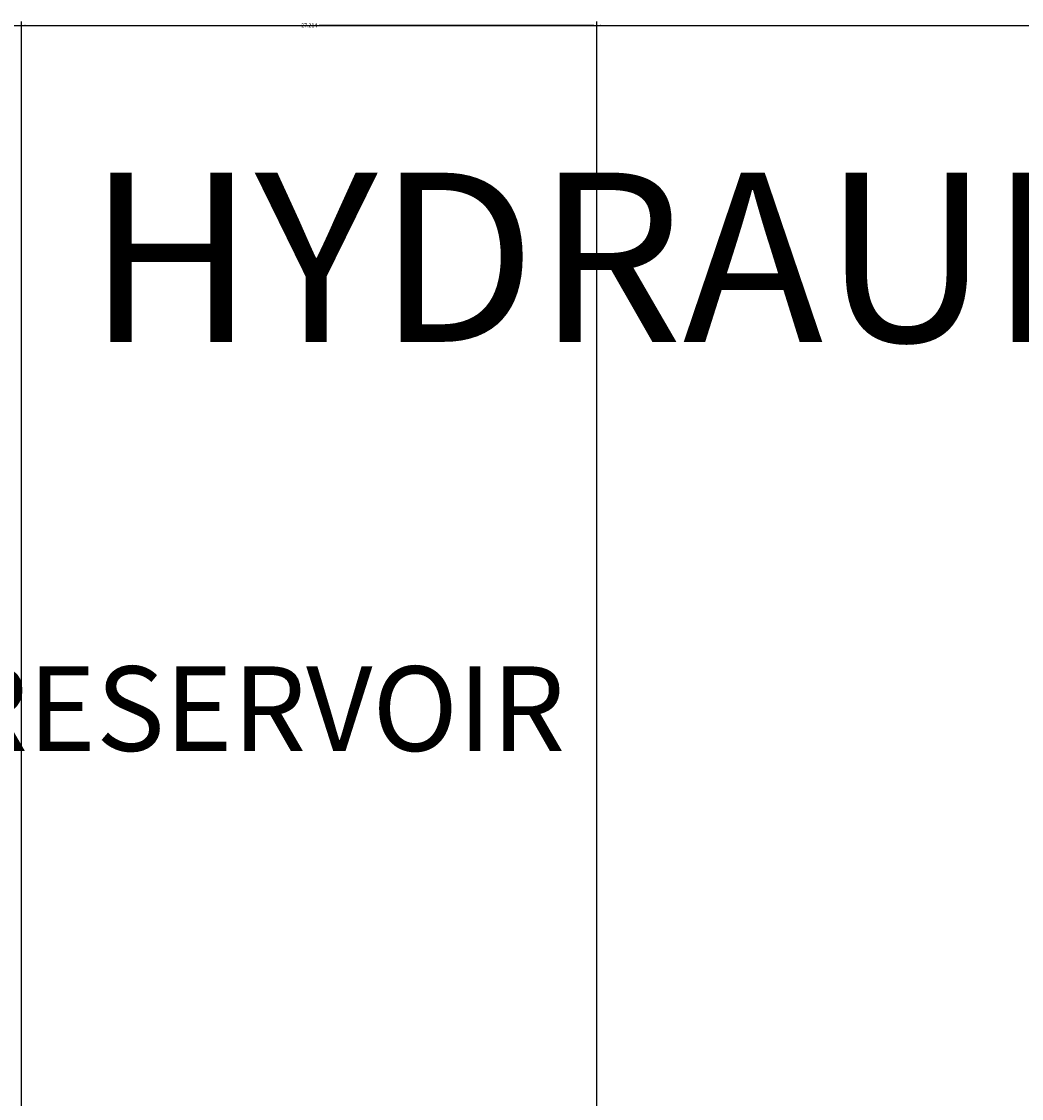
# Model space of a CAD drawing. Units: millimetres. Extents: x -11 to 280, y -4 to 208.
# Tile 46 of 55: x 91 to 139, y 157 to 208. Entities that reach past the tile are written whole.
import ezdxf
from ezdxf import colors
from ezdxf.entities.mleader import LeaderData, LeaderLine
from ezdxf.math import Vec2, Vec3

# ---------------------------------------------------------------- set-up
doc = ezdxf.new("R2010")
doc.units = ezdxf.units.MM
doc.layers.add('M-ANNO-TEXT', color=7, linetype='Continuous', lineweight=18)
doc.layers.add('M-DIMS', color=2, linetype='Continuous', lineweight=18)
doc.styles.get("Standard").update_dxf_attribs({"font": 'arial.ttf'})
doc.dimstyles.get("Standard").update_dxf_attribs({"dimtxt": 0.18, "dimasz": 0.18, "dimexe": 0.18, "dimexo": 0.0625, "dimgap": 0.09, "dimtad": 0, "dimtih": 1, "dimtoh": 1, "dimdec": 4, "dimzin": 0, "dimdsep": 46, "dimtxsty": 'Standard', "dimcen": 0.09, "dimadec": 0, "dimazin": 0, "dimtfac": 1, "dimtdec": 4, "dimtofl": 0, "dimtmove": 0, "dimatfit": 3, "dimfxl": 1, "dimtolj": 1, "dimtzin": 0, "dimarcsym": 0})

# ---------------------------------------------------------------- blocks, each defined once
blk = doc.blocks.new('*D5')
at = {"layer": 'Defpoints', "color": 0, "transparency": 16777216}
for p in [(24.759, 192.645), (-10.087, 11.435), (261.686, 11.435)]:
    blk.add_point(p, dxfattribs=at)
at = {"layer": 'M-DIMS', "color": 0, "lineweight": -2, "transparency": 16777216}
for p, q in [((24.696, 192.645), (-10.267, 192.645)), ((-10.087, 192.465), (-10.087, 102.222)), ((-10.087, 11.615), (-10.087, 101.858)), ((261.624, 11.435), (-10.267, 11.435))]:
    blk.add_line(p, q, dxfattribs=at)
at = {"layer": 'M-DIMS', "color": 0, "transparency": 16777216}
for points in [[(-10.117, 192.465), (-10.057, 192.465), (-10.087, 192.645)], [(-10.117, 11.615), (-10.057, 11.615), (-10.087, 11.435)]]:
    blk.add_solid(points, dxfattribs=at)
at = {"layer": 'M-DIMS', "color": 0, "transparency": 16777216, "insert": (-10.087, 102.04), "char_height": 0.18, "attachment_point": 5}
blk.add_mtext('\\A1;181.2', dxfattribs=at)
blk = doc.blocks.new('*D6')
at = {"layer": 'Defpoints', "color": 0, "transparency": 16777216}
for p in [(236.935, 207.495), (66.388, 179.241), (236.935, 165.103)]:
    blk.add_point(p, dxfattribs=at)
at = {"layer": 'M-DIMS', "color": 0, "lineweight": -2, "transparency": 16777216}
for p, q in [((66.388, 179.304), (66.388, 207.675)), ((66.568, 207.495), (151.206, 207.495)), ((236.755, 207.495), (152.117, 207.495)), ((236.935, 165.166), (236.935, 207.675))]:
    blk.add_line(p, q, dxfattribs=at)
at = {"layer": 'M-DIMS', "color": 0, "transparency": 16777216}
for points in [[(66.568, 207.525), (66.568, 207.465), (66.388, 207.495)], [(236.755, 207.525), (236.755, 207.465), (236.935, 207.495)]]:
    blk.add_solid(points, dxfattribs=at)
at = {"layer": 'M-DIMS', "color": 0, "transparency": 16777216, "insert": (151.661, 207.495), "char_height": 0.18, "attachment_point": 5}
blk.add_mtext('\\A1;170.55', dxfattribs=at)
blk = doc.blocks.new('*D11')
at = {"layer": 'Defpoints', "color": 0, "transparency": 16777216}
for p in [(118.514, 207.495), (91.3, 98.149), (118.514, 96.485)]:
    blk.add_point(p, dxfattribs=at)
at = {"layer": 'M-DIMS', "color": 0, "lineweight": -2, "transparency": 16777216}
for p, q in [((91.3, 98.212), (91.3, 207.675)), ((91.48, 207.495), (104.442, 207.495)), ((118.334, 207.495), (105.372, 207.495)), ((118.514, 96.547), (118.514, 207.675))]:
    blk.add_line(p, q, dxfattribs=at)
at = {"layer": 'M-DIMS', "color": 0, "transparency": 16777216}
for points in [[(91.48, 207.525), (91.48, 207.465), (91.3, 207.495)], [(118.334, 207.525), (118.334, 207.465), (118.514, 207.495)]]:
    blk.add_solid(points, dxfattribs=at)
at = {"layer": 'M-DIMS', "color": 0, "transparency": 16777216, "insert": (104.907, 207.495), "char_height": 0.18, "attachment_point": 5}
blk.add_mtext('\\A1;27.214', dxfattribs=at)
blk = doc.blocks.new('*D12')
at = {"layer": 'Defpoints', "color": 0, "transparency": 16777216}
for p in [(173.804, 207.495), (118.514, 96.485), (173.804, 89.387)]:
    blk.add_point(p, dxfattribs=at)
at = {"layer": 'M-DIMS', "color": 0, "lineweight": -2, "transparency": 16777216}
for p, q in [((118.514, 96.547), (118.514, 207.675)), ((118.694, 207.495), (145.765, 207.495)), ((173.624, 207.495), (146.553, 207.495)), ((173.804, 89.45), (173.804, 207.675))]:
    blk.add_line(p, q, dxfattribs=at)
at = {"layer": 'M-DIMS', "color": 0, "transparency": 16777216}
for points in [[(118.694, 207.525), (118.694, 207.465), (118.514, 207.495)], [(173.624, 207.525), (173.624, 207.465), (173.804, 207.495)]]:
    blk.add_solid(points, dxfattribs=at)
at = {"layer": 'M-DIMS', "color": 0, "transparency": 16777216, "insert": (146.159, 207.495), "char_height": 0.18, "attachment_point": 5}
blk.add_mtext('\\A1;55.29', dxfattribs=at)

msp = doc.modelspace()

# ---------------------------------------------------------------- texts
at = {"layer": 'M-ANNO-TEXT', "insert": (94.3946, 200.5299), "char_height": 8, "attachment_point": 1}
msp.add_mtext_dynamic_manual_height_columns('HYDRAULIC SYSTEM ', width=219.105197, gutter_width=12.5, heights=[0], dxfattribs=at)

# ---------------------------------------------------------------- dimensions: what is measured, and where the dimension line sits
at = {"layer": 'M-DIMS'}
for base, p1, p2, override, picture, middle in [((236.9353, 207.495), (66.3875, 179.2412), (236.9353, 165.103), {"dimdec": 2, "dimlfac": 1, "dimrnd": 0, "dimzin": 0, "dimdsep": 46, "dimlunit": 2}, '*D6', (151.6614, 207.495)), ((118.5137, 207.495), (91.3, 98.1491), (118.5137, 96.4849), {"dimdec": 3, "dimlfac": 1, "dimrnd": 0, "dimzin": 0, "dimdsep": 46, "dimlunit": 2}, '*D11', (104.9068, 207.495)), ((173.8038, 207.495), (118.5137, 96.4849), (173.8038, 89.3873), {"dimdec": 2, "dimlfac": 1, "dimrnd": 0, "dimzin": 0, "dimdsep": 46, "dimlunit": 2}, '*D12', (146.1587, 207.495))]:
    dim = msp.add_linear_dim(base=base, p1=p1, p2=p2, dimstyle='Standard', override=override, dxfattribs=at)
    dim.commit()
    dim.dimension.update_dxf_attribs({"geometry": picture, "text_midpoint": middle})
dim = msp.add_linear_dim(base=(-10.0865, 11.4346), p1=(24.7588, 192.645), p2=(261.6863, 11.4346), angle=90, dimstyle='Standard', override={"dimdec": 1, "dimlfac": 1, "dimrnd": 0, "dimzin": 0, "dimdsep": 46, "dimlunit": 2}, dxfattribs=at)
dim.commit()
dim.dimension.update_dxf_attribs({"geometry": '*D5', "text_midpoint": (-10.0865, 102.0398)})

# ---------------------------------------------------------------- leaders
at = {"layer": 'M-ANNO-TEXT'}
ml = msp.add_multileader_mtext('Standard', dxfattribs=at)
ml.set_content('RESERVOIR', color=256)
ml.set_leader_properties()
ml.build(insert=Vec2(0, 0))
ctx = ml.context
ctx.base_point, ctx.plane_origin = Vec3(86.1452, 175.1554), Vec3(66.3875, 168.3671)
notes = []
notes.append((ctx, [(0, (1, 1, 0), (78.1452, 175.1554), (1, 0), 8, [(0, [(66.3875, 168.3671)], 0, [])])]))
ctx.mtext.insert, ctx.mtext.flow_direction = Vec3(88.1452, 177.1895), 5
for ctx, leaders in notes:
    for number, flags, end, landing, length, lines in leaders:
        leader = LeaderData()
        leader.index, (leader.has_last_leader_line, leader.has_dogleg_vector, leader.attachment_direction) = number, flags
        leader.last_leader_point, leader.dogleg_vector, leader.dogleg_length = Vec3(end), Vec3(landing), length
        for number, points, colour, breaks in lines:
            line = LeaderLine()
            line.index, line.vertices, line.color, line.breaks = number, Vec3.list(points), colors.encode_raw_color(colour), breaks
            leader.lines.append(line)
        ctx.leaders.append(leader)

doc.saveas('drawing.dxf')
